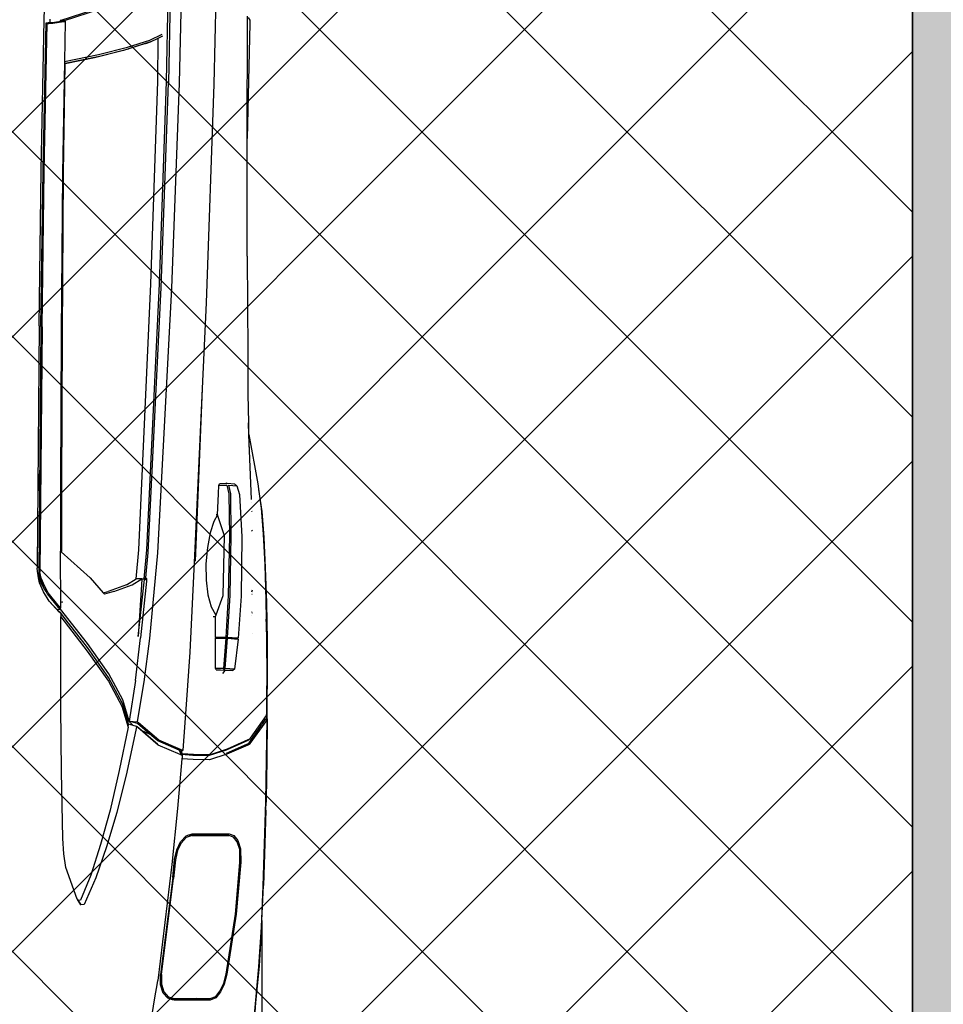
# Model space of a CAD drawing. Units: inches. Extents: x 2167 to 2589, y 1680 to 2489.
# Tile 18 of 38: x 2387 to 2419, y 1727 to 1761. Entities that reach past the tile are written whole.
import ezdxf

# ---------------------------------------------------------------- set-up
doc = ezdxf.new("R2010")
doc.units = ezdxf.units.IN
doc.header["$MEASUREMENT"] = 0
doc.layers.get('0').update_dxf_attribs({"color": 250})
doc.layers.add('A-FLOR-PATT', color=254, linetype='Continuous', lineweight=13, true_color=0xfeeab9)
for name, color, linetype, lineweight in [('C-PRKG-VEHS', 8, 'Continuous', 13), ('L-PVMT-PATT', 252, 'Continuous', 13), ('walls', 7, 'Continuous', 35)]:
    doc.layers.add(name, color=color, linetype=linetype, lineweight=lineweight)
doc.layers.add('Edges', color=250, linetype='Continuous')

# ---------------------------------------------------------------- blocks, each defined once
blk = doc.blocks.new('Nissan Qashqai pl')
at = {"layer": 'Edges'}
for p, q in [((10.4573, 12.8093), (10.4889, 12.8119)), ((10.4613, 12.8099), (10.4926, 12.8125)), ((10.4889, 12.8119), (10.526, 12.8138)), ((10.4926, 12.8125), (10.5294, 12.8143)), ((10.526, 12.8138), (10.569, 12.8151)), ((10.5294, 12.8143), (10.5719, 12.8156)), ((10.569, 12.8151), (10.5919, 12.8155)), ((10.5719, 12.8156), (10.6176, 12.8164)), ((10.5919, 12.8155), (10.6151, 12.8159)), ((10.5981, 12.8157), (10.5919, 12.8155)), ((10.6174, 12.816), (10.5981, 12.8157)), ((10.6151, 12.8159), (10.6644, 12.8162)), ((10.6176, 12.8164), (10.6651, 12.8167)), ((10.6644, 12.8162), (10.7078, 12.8159)), ((10.6651, 12.8167), (10.666, 12.8167)), ((10.666, 12.8167), (10.677, 12.8167)), ((10.6729, 12.8157), (10.7082, 12.8156)), ((10.6809, 12.8167), (10.677, 12.8167)), ((10.7128, 12.8166), (10.6809, 12.8167)), ((10.7078, 12.8159), (10.7083, 12.8156)), ((10.7082, 12.8156), (10.7078, 12.8159)), ((10.7085, 12.8153), (10.7082, 12.8156)), ((10.7082, 12.8156), (10.7083, 12.8156)), ((10.7083, 12.8156), (10.7087, 12.8153)), ((10.7083, 12.8156), (10.7125, 12.8156)), ((10.7087, 12.8153), (10.7363, 12.7959)), ((10.7139, 12.8164), (10.7125, 12.8156)), ((10.7137, 12.8148), (10.7125, 12.8156)), ((10.7128, 12.8166), (10.7625, 12.8161)), ((10.7128, 12.8166), (10.724, 12.8166)), ((10.7137, 12.8148), (10.7138, 12.8147)), ((10.7418, 12.7947), (10.7138, 12.8147)), ((10.7139, 12.8164), (10.7148, 12.8157)), ((10.7628, 12.8158), (10.7139, 12.8164)), ((10.7148, 12.8157), (10.7429, 12.7956)), ((10.7685, 12.8161), (10.724, 12.8166)), ((10.7625, 12.8161), (10.7628, 12.8161)), ((10.7628, 12.8161), (10.8099, 12.8152)), ((10.8131, 12.8149), (10.7628, 12.8158)), ((10.7688, 12.8161), (10.7685, 12.8161)), ((10.8099, 12.8152), (10.7688, 12.8161)), ((10.8099, 12.8152), (10.8131, 12.8152)), ((10.8134, 12.8152), (10.8131, 12.8152)), ((10.8644, 12.8135), (10.8131, 12.8149)), ((10.8134, 12.8152), (10.8142, 12.8152)), ((10.8142, 12.8152), (10.8142, 12.8152)), ((10.8237, 12.8149), (10.8142, 12.8152)), ((10.8237, 12.8149), (10.864, 12.8138)), ((10.8596, 12.8138), (10.8589, 12.8138)), ((10.8642, 12.8136), (10.8596, 12.8138)), ((10.864, 12.8138), (10.8642, 12.8138)), ((10.8642, 12.8138), (10.9152, 12.812)), ((10.9158, 12.8118), (10.8644, 12.8135)), ((10.9577, 12.8101), (10.9152, 12.812)), ((10.9657, 12.8095), (10.9158, 12.8118)), ((10.3679, 12.7944), (10.4275, 12.8051)), ((10.4275, 12.8051), (10.4304, 12.8056)), ((10.4304, 12.8056), (10.4339, 12.8061)), ((10.4339, 12.8061), (10.4573, 12.8093)), ((10.4339, 12.8061), (10.4345, 12.8062)), ((10.4345, 12.8062), (10.4613, 12.8099)), ((10.9577, 12.8101), (10.9649, 12.8097)), ((10.9577, 12.8101), (11.1283, 12.8101)), ((10.9649, 12.8097), (11.0127, 12.8067)), ((11.0138, 12.8064), (10.9657, 12.8095)), ((11.0127, 12.8067), (11.0576, 12.8026)), ((11.059, 12.8023), (11.0138, 12.8064)), ((11.0576, 12.8026), (11.0798, 12.8008)), ((11.0768, 12.8008), (11.059, 12.8023)), ((9.8643, 12.7927), (9.8598, 12.7928)), ((9.8614, 12.7937), (9.8647, 12.7956)), ((10.0085, 12.7922), (9.8643, 12.7927)), ((9.8647, 12.7956), (9.869, 12.7954)), ((9.869, 12.7954), (10.0085, 12.7922)), ((10.0124, 12.7922), (10.0085, 12.7922)), ((10.1513, 12.7924), (10.0124, 12.7922)), ((10.1513, 12.7924), (10.2677, 12.793)), ((10.2677, 12.793), (10.3189, 12.7931)), ((10.3189, 12.7931), (10.3537, 12.7939)), ((10.3537, 12.7939), (10.3832, 12.7945)), ((10.3679, 12.7944), (10.3537, 12.7939)), ((10.4468, 12.7976), (10.3679, 12.7944)), ((10.4503, 12.7976), (10.4502, 12.7976)), ((10.4603, 12.7976), (10.4613, 12.7978)), ((10.4838, 12.7977), (10.4852, 12.7982)), ((10.5565, 12.7985), (10.5591, 12.7977)), ((10.5615, 12.7978), (10.5617, 12.7985)), ((10.583, 12.7984), (10.5834, 12.798)), ((10.5836, 12.798), (10.5831, 12.7984)), ((10.5847, 12.798), (10.5841, 12.7984)), ((10.5873, 12.7981), (10.5873, 12.7981)), ((10.6087, 12.7983), (10.6087, 12.7984)), ((10.7363, 12.7959), (10.7376, 12.795)), ((10.7387, 12.794), (10.7376, 12.795)), ((10.7376, 12.795), (10.7378, 12.7946)), ((10.7378, 12.7946), (10.7379, 12.7945)), ((10.7378, 12.7946), (10.7385, 12.7932)), ((10.7385, 12.7932), (10.7497, 12.7679)), ((10.7387, 12.794), (10.7396, 12.7922)), ((10.7396, 12.7922), (10.7507, 12.7669)), ((10.743, 12.7939), (10.7418, 12.7947)), ((10.7432, 12.7954), (10.7426, 12.7954)), ((10.7429, 12.7956), (10.7432, 12.7954)), ((10.7434, 12.793), (10.743, 12.7939)), ((10.7441, 12.7954), (10.7432, 12.7954)), ((10.7432, 12.7954), (10.744, 12.7948)), ((10.7437, 12.7921), (10.7434, 12.793)), ((10.7438, 12.7921), (10.7437, 12.7921)), ((10.7438, 12.7921), (10.7549, 12.7666)), ((10.744, 12.7948), (10.7448, 12.793)), ((10.7448, 12.793), (10.7559, 12.7674)), ((10.4282, 12.7775), (10.4274, 12.7679)), ((10.4282, 12.7775), (10.4299, 12.7798)), ((10.4291, 12.77), (10.4299, 12.7798)), ((10.4299, 12.7798), (10.4406, 12.7829)), ((10.4406, 12.7829), (10.4919, 12.7858)), ((10.4919, 12.7858), (10.564, 12.7851)), ((10.564, 12.7851), (10.6151, 12.7813)), ((10.615, 12.7803), (10.6142, 12.7686)), ((10.6151, 12.7813), (10.615, 12.7803)), ((10.615, 12.7676), (10.6151, 12.7803)), ((10.6151, 12.7803), (10.615, 12.7803)), ((10.6151, 12.7803), (10.6151, 12.7813)), ((10.6151, 12.7685), (10.616, 12.7812)), ((10.616, 12.7812), (10.6526, 12.7768)), ((10.6526, 12.7768), (10.6518, 12.7657)), ((10.6526, 12.7768), (10.6543, 12.7749)), ((10.8523, 12.7704), (10.8546, 12.7762)), ((10.8546, 12.7762), (10.8607, 12.7808)), ((10.8622, 12.7801), (10.8565, 12.7757)), ((10.8607, 12.7808), (10.8708, 12.7841)), ((10.8716, 12.7832), (10.8622, 12.7801)), ((10.8708, 12.7841), (10.8869, 12.7844)), ((10.887, 12.7835), (10.8716, 12.7832)), ((10.8869, 12.7844), (10.9499, 12.7789)), ((10.9498, 12.7781), (10.887, 12.7835)), ((11.0226, 12.7668), (10.9498, 12.7781)), ((10.9499, 12.7789), (11.0229, 12.7676)), ((10.4263, 12.7665), (10.4274, 12.7674)), ((10.4274, 12.7679), (10.4274, 12.7674)), ((10.4274, 12.7674), (10.4275, 12.7586)), ((10.4398, 12.7724), (10.4291, 12.77)), ((10.4291, 12.7677), (10.4398, 12.7701)), ((10.4293, 12.7579), (10.4291, 12.7677)), ((10.4909, 12.773), (10.4398, 12.7724)), ((10.4398, 12.7701), (10.4909, 12.7708)), ((10.4908, 12.7648), (10.4653, 12.7564)), ((10.563, 12.7633), (10.4908, 12.7648)), ((10.5631, 12.7715), (10.4909, 12.773)), ((10.4909, 12.7708), (10.563, 12.7692)), ((10.563, 12.7692), (10.6142, 12.7663)), ((10.6142, 12.7686), (10.5631, 12.7715)), ((10.6142, 12.766), (10.6141, 12.7537)), ((10.6142, 12.7686), (10.6142, 12.7677)), ((10.6142, 12.7677), (10.615, 12.7676)), ((10.6142, 12.7677), (10.6142, 12.7663)), ((10.6142, 12.7663), (10.6142, 12.766)), ((10.6151, 12.7676), (10.615, 12.7676)), ((10.615, 12.7537), (10.6151, 12.7659)), ((10.6518, 12.7657), (10.6151, 12.7685)), ((10.6151, 12.7676), (10.6151, 12.7685)), ((10.6151, 12.7662), (10.6151, 12.7676)), ((10.6151, 12.7662), (10.6518, 12.7634)), ((10.6151, 12.7659), (10.6151, 12.7662)), ((10.6536, 12.7639), (10.6518, 12.7657)), ((10.6518, 12.7657), (10.6518, 12.7634)), ((10.6518, 12.7634), (10.6536, 12.7639)), ((10.6543, 12.7656), (10.6535, 12.7546)), ((10.6535, 12.7546), (10.6536, 12.7639)), ((10.6536, 12.7639), (10.6537, 12.7658)), ((10.6537, 12.7658), (10.6543, 12.7749)), ((10.6537, 12.7658), (10.6543, 12.7656)), ((10.6543, 12.7749), (10.6543, 12.7656)), ((10.6578, 12.7628), (10.6543, 12.7656)), ((10.7497, 12.7679), (10.7565, 12.7473)), ((10.7507, 12.7669), (10.7575, 12.7462)), ((10.7559, 12.7674), (10.7626, 12.7467)), ((10.8523, 12.7255), (10.8523, 12.7704)), ((10.8543, 12.7702), (10.8538, 12.753)), ((10.8565, 12.7757), (10.8543, 12.7702)), ((10.8543, 12.7255), (10.8543, 12.7702)), ((11.0339, 12.7639), (11.0226, 12.7668)), ((11.0229, 12.7676), (11.0348, 12.7645)), ((11.0429, 12.7597), (11.0339, 12.7639)), ((11.0348, 12.7645), (11.0444, 12.7601)), ((9.8024, 12.7549), (9.9426, 12.7518)), ((10.4293, 12.7579), (10.4275, 12.7586)), ((10.4398, 12.7573), (10.4293, 12.7579)), ((10.4653, 12.7564), (10.4398, 12.7573)), ((10.4653, 12.7561), (10.4652, 12.7545)), ((10.4653, 12.7564), (10.4653, 12.7561)), ((10.4653, 12.7564), (10.4653, 12.7564)), ((10.4653, 12.7564), (10.4653, 12.7561)), ((10.4653, 12.7561), (10.4653, 12.7561)), ((10.4653, 12.7561), (10.4732, 12.7517)), ((10.5867, 12.7545), (10.563, 12.7633)), ((10.5769, 12.7484), (10.5863, 12.7537)), ((10.5863, 12.7537), (10.5867, 12.7545)), ((10.5885, 12.7538), (10.5867, 12.7545)), ((10.5885, 12.751), (10.5885, 12.7538)), ((10.6141, 12.7537), (10.5885, 12.7538)), ((10.6141, 12.7537), (10.615, 12.7537)), ((10.6517, 12.754), (10.615, 12.7537)), ((10.6518, 12.7634), (10.6517, 12.754)), ((10.6535, 12.7546), (10.6517, 12.754)), ((10.8528, 12.7503), (10.8535, 12.7521)), ((10.8535, 12.7521), (10.8538, 12.753)), ((10.8538, 12.7521), (10.8535, 12.7521)), ((10.8538, 12.753), (10.8538, 12.7521)), ((10.8538, 12.7521), (10.8538, 12.7502)), ((11.0497, 12.7542), (11.0429, 12.7597)), ((11.0444, 12.7601), (11.0516, 12.7542)), ((11.0523, 12.7475), (11.0497, 12.7542)), ((11.0516, 12.7542), (11.0543, 12.7473)), ((9.9426, 12.7518), (10.2081, 12.7424)), ((10.2081, 12.7424), (10.312, 12.7377)), ((10.4732, 12.7517), (10.4871, 12.7474)), ((10.4871, 12.7474), (10.5048, 12.744)), ((10.5048, 12.744), (10.5246, 12.7423)), ((10.5246, 12.7423), (10.5445, 12.7425)), ((10.5445, 12.7425), (10.5625, 12.7446)), ((10.5625, 12.7446), (10.5769, 12.7484)), ((10.7565, 12.7473), (10.7563, 12.7273)), ((10.7575, 12.7462), (10.7572, 12.7263)), ((10.7626, 12.7467), (10.7623, 12.7269)), ((10.8528, 12.742), (10.8528, 12.7503)), ((10.8528, 12.742), (10.8538, 12.742)), ((10.8528, 12.7419), (10.8528, 12.742)), ((10.8538, 12.7419), (10.8528, 12.7419)), ((10.8528, 12.7242), (10.8528, 12.7419)), ((10.8538, 12.7502), (10.8538, 12.742)), ((10.8538, 12.742), (10.8538, 12.7419)), ((10.8538, 12.7214), (10.8538, 12.7419)), ((11.0528, 12.73), (11.0523, 12.7475)), ((11.0523, 12.7312), (11.0523, 12.7475)), ((11.0543, 12.7473), (11.0543, 12.7035)), ((10.312, 12.7377), (10.5214, 12.7293)), ((10.312, 12.7377), (10.5147, 12.7285)), ((10.5147, 12.7285), (10.6318, 12.7228)), ((11.0523, 12.7312), (11.0528, 12.73)), ((11.0523, 12.7287), (11.0523, 12.7312)), ((11.0528, 12.7274), (11.0523, 12.7287)), ((11.0523, 12.7037), (11.0523, 12.7287)), ((11.0528, 12.7274), (11.0528, 12.73)), ((11.0528, 12.73), (11.0538, 12.7273)), ((10.6318, 12.7228), (10.6955, 12.7184)), ((10.6955, 12.7184), (10.7509, 12.714)), ((10.7563, 12.7273), (10.7553, 12.7134)), ((10.7572, 12.7263), (10.7563, 12.7126)), ((10.7623, 12.7269), (10.7615, 12.7131)), ((10.8528, 12.7242), (10.8523, 12.7255)), ((10.8538, 12.7214), (10.8528, 12.7242)), ((10.855, 12.7181), (10.8538, 12.7214)), ((10.8543, 12.7255), (10.8569, 12.7184)), ((10.8622, 12.7114), (10.855, 12.7181)), ((10.8569, 12.7184), (10.8637, 12.712)), ((11.0528, 12.7274), (11.0528, 12.6985)), ((11.0538, 12.7273), (11.0538, 12.7018)), ((9.9414, 12.71), (9.8143, 12.713)), ((10.19, 12.7008), (9.9414, 12.71)), ((10.7501, 12.7114), (10.7387, 12.6849)), ((10.7507, 12.7098), (10.7397, 12.684)), ((10.7563, 12.7109), (10.7449, 12.6843)), ((10.7507, 12.7132), (10.7501, 12.7114)), ((10.7506, 12.7111), (10.7507, 12.7132)), ((10.7507, 12.7132), (10.7509, 12.714)), ((10.751, 12.7132), (10.7507, 12.7132)), ((10.7511, 12.7107), (10.7507, 12.7098)), ((10.7524, 12.7106), (10.7507, 12.7098)), ((10.7522, 12.7131), (10.7509, 12.714)), ((10.7516, 12.7131), (10.7509, 12.714)), ((10.7519, 12.7128), (10.7511, 12.7107)), ((10.7522, 12.7131), (10.7516, 12.7131)), ((10.7519, 12.7128), (10.7516, 12.7131)), ((10.7526, 12.7124), (10.7519, 12.7128)), ((10.7553, 12.7134), (10.7522, 12.7131)), ((10.7524, 12.7106), (10.7526, 12.7124)), ((10.7556, 12.7122), (10.7524, 12.7106)), ((10.7526, 12.7124), (10.7526, 12.7127)), ((10.7532, 12.712), (10.7526, 12.7124)), ((10.7556, 12.7122), (10.7532, 12.712)), ((10.7561, 12.7125), (10.7556, 12.7122)), ((10.7561, 12.7125), (10.7563, 12.7126)), ((10.7563, 12.7125), (10.7561, 12.7125)), ((10.7563, 12.7123), (10.7561, 12.7123)), ((10.7563, 12.7126), (10.7573, 12.7135)), ((10.7563, 12.7126), (10.7563, 12.7125)), ((10.7569, 12.7125), (10.7563, 12.7109)), ((10.7569, 12.7125), (10.7563, 12.7125)), ((10.7563, 12.7125), (10.7563, 12.7123)), ((10.7573, 12.7135), (10.7569, 12.7125)), ((10.7573, 12.7135), (10.7604, 12.7132)), ((10.7604, 12.7132), (10.7615, 12.7131)), ((10.7615, 12.7131), (10.8218, 12.7077)), ((10.8218, 12.7077), (10.8896, 12.7008)), ((10.8718, 12.7068), (10.8622, 12.7114)), ((10.8637, 12.712), (10.8727, 12.7077)), ((10.8836, 12.7041), (10.8718, 12.7068)), ((10.8727, 12.7077), (10.8839, 12.7051)), ((10.9054, 12.702), (10.8836, 12.7041)), ((10.8839, 12.7051), (10.9067, 12.7029)), ((9.8101, 12.6993), (9.9411, 12.6966)), ((9.9393, 12.6944), (9.8119, 12.697)), ((10.1849, 12.6857), (9.9393, 12.6944)), ((10.1894, 12.6879), (9.9411, 12.6966)), ((10.5113, 12.6839), (10.19, 12.7008)), ((10.8896, 12.7008), (11.0304, 12.6838)), ((10.9054, 12.702), (11.0232, 12.6871)), ((11.0231, 12.6882), (10.9067, 12.7029)), ((11.0443, 12.6911), (11.0501, 12.6964)), ((11.052, 12.6958), (11.0458, 12.6903)), ((11.0501, 12.6964), (11.0523, 12.7037)), ((11.0528, 12.6985), (11.052, 12.6958)), ((11.0538, 12.7018), (11.0528, 12.6985)), ((11.0543, 12.7035), (11.0538, 12.7018)), ((9.8891, 12.6741), (9.8818, 12.6891)), ((9.8867, 12.6842), (9.8838, 12.6901)), ((9.9393, 12.684), (9.8867, 12.6842)), ((9.8911, 12.675), (9.8867, 12.6842)), ((10.1849, 12.6754), (9.9393, 12.684)), ((10.5079, 12.6703), (10.1849, 12.6857)), ((10.5109, 12.6721), (10.1894, 12.6879)), ((10.6152, 12.674), (10.5113, 12.6839)), ((10.7387, 12.6849), (10.7177, 12.6604)), ((10.7449, 12.6843), (10.7232, 12.6594)), ((10.7438, 12.6836), (10.7265, 12.6635)), ((10.7397, 12.684), (10.7334, 12.6766)), ((11.0231, 12.6882), (11.035, 12.6883)), ((11.0358, 12.6872), (11.0232, 12.6871)), ((11.0357, 12.6829), (11.0304, 12.6838)), ((11.035, 12.6883), (11.0443, 12.6911)), ((11.0491, 12.6807), (11.0357, 12.6829)), ((11.0458, 12.6903), (11.0358, 12.6872)), ((11.0449, 12.6812), (11.0448, 12.6812)), ((11.0492, 12.6807), (11.0491, 12.6807)), ((11.1336, 12.667), (11.0492, 12.6807)), ((9.8978, 12.6472), (9.8891, 12.6741)), ((9.8911, 12.6749), (9.8911, 12.675)), ((9.8931, 12.6691), (9.8911, 12.6749)), ((9.8911, 12.6749), (9.8998, 12.6481)), ((9.8931, 12.669), (9.8931, 12.6691)), ((9.8931, 12.669), (9.9018, 12.6421)), ((10.5079, 12.6607), (10.1849, 12.6754)), ((10.543, 12.6671), (10.5079, 12.6703)), ((10.5417, 12.6693), (10.5109, 12.6721)), ((10.5417, 12.6693), (10.5427, 12.6702)), ((10.5417, 12.6693), (10.543, 12.6671)), ((10.5436, 12.6687), (10.5427, 12.6702)), ((10.5427, 12.6702), (10.5458, 12.67)), ((10.544, 12.6678), (10.5436, 12.6687)), ((10.5458, 12.67), (10.6144, 12.6629)), ((10.6678, 12.6672), (10.6152, 12.674)), ((10.7334, 12.6766), (10.7186, 12.6593)), ((10.7265, 12.6635), (10.7316, 12.6741)), ((10.543, 12.6576), (10.5079, 12.6607)), ((10.544, 12.6678), (10.543, 12.6671)), ((10.543, 12.6646), (10.543, 12.6671)), ((10.543, 12.6646), (10.543, 12.6576)), ((10.5439, 12.6646), (10.543, 12.6646)), ((10.5502, 12.6526), (10.543, 12.6646)), ((10.5502, 12.6456), (10.543, 12.6576)), ((10.5439, 12.6646), (10.613, 12.6601)), ((10.547, 12.6674), (10.544, 12.6678)), ((10.613, 12.6601), (10.547, 12.6674)), ((10.6664, 12.6566), (10.6144, 12.6629)), ((10.6664, 12.6566), (10.7155, 12.649)), ((10.7137, 12.6595), (10.6678, 12.6672)), ((10.7165, 12.6591), (10.7137, 12.6595)), ((10.7186, 12.6593), (10.7155, 12.649)), ((10.7155, 12.649), (10.7165, 12.6591)), ((10.7177, 12.6604), (10.7165, 12.6591)), ((10.7221, 12.6581), (10.7209, 12.654)), ((10.7232, 12.6594), (10.7221, 12.6581)), ((10.7221, 12.6581), (10.7224, 12.6587)), ((10.7221, 12.6581), (10.7247, 12.6575)), ((10.7265, 12.6635), (10.7224, 12.6587)), ((10.7247, 12.6575), (10.7776, 12.646)), ((9.9066, 12.6119), (9.8978, 12.6472)), ((9.9086, 12.6129), (9.8998, 12.6481)), ((10.5584, 12.6306), (10.5502, 12.6526)), ((10.5502, 12.6456), (10.5584, 12.6236)), ((10.7155, 12.649), (10.69, 12.6414)), ((10.7155, 12.6473), (10.6943, 12.641)), ((10.6976, 12.6401), (10.7228, 12.6477)), ((10.7209, 12.654), (10.7155, 12.6485)), ((10.7155, 12.649), (10.7155, 12.6485)), ((10.7155, 12.6485), (10.7155, 12.6473)), ((10.7192, 12.6484), (10.7155, 12.6473)), ((10.7209, 12.654), (10.7192, 12.6484)), ((10.7228, 12.6477), (10.7192, 12.6484)), ((10.7228, 12.6477), (10.7754, 12.637)), ((10.7776, 12.646), (10.8264, 12.6341)), ((9.9018, 12.6421), (9.9106, 12.6068)), ((10.69, 12.6414), (10.6583, 12.6245)), ((10.6943, 12.641), (10.6627, 12.6241)), ((10.6671, 12.6238), (10.6976, 12.6401)), ((10.7754, 12.637), (10.8239, 12.6261)), ((10.8264, 12.6341), (10.8682, 12.6216)), ((10.5584, 12.6306), (10.5617, 12.619)), ((10.56, 12.6176), (10.5584, 12.6236)), ((10.6583, 12.6245), (10.6215, 12.5986)), ((10.6627, 12.6241), (10.6261, 12.5984)), ((10.6306, 12.5982), (10.6671, 12.6238)), ((10.8239, 12.6261), (10.8653, 12.6144)), ((10.8682, 12.6216), (10.9059, 12.6087)), ((9.8652, 12.5704), (9.8516, 12.6129)), ((9.9149, 12.5705), (9.9066, 12.6119)), ((9.9169, 12.5714), (9.9086, 12.6129)), ((10.5419, 12.6018), (10.56, 12.6176)), ((10.56, 12.6176), (10.5617, 12.619)), ((10.8653, 12.6144), (10.9026, 12.6025)), ((10.9059, 12.6087), (10.9384, 12.5945)), ((9.8652, 12.5654), (9.8516, 12.6079)), ((9.9106, 12.6068), (9.9177, 12.5714)), ((10.51, 12.5666), (10.5419, 12.6018)), ((10.6215, 12.5986), (10.5796, 12.5655)), ((10.5892, 12.5659), (10.6306, 12.5982)), ((10.6261, 12.5984), (10.593, 12.5726)), ((10.9026, 12.6025), (10.933, 12.5901)), ((10.9316, 12.586), (10.8932, 12.572)), ((10.9316, 12.586), (10.9334, 12.5872)), ((10.932, 12.5862), (10.9316, 12.586)), ((10.9335, 12.5871), (10.932, 12.5862)), ((10.933, 12.5901), (10.9334, 12.5872)), ((10.9334, 12.5872), (10.9386, 12.5905)), ((10.9334, 12.5872), (10.9335, 12.5871)), ((10.9386, 12.5905), (10.9335, 12.5871)), ((10.9384, 12.5945), (10.9386, 12.5905)), ((9.8652, 12.5706), (9.8664, 12.5714)), ((9.8652, 12.5706), (9.8665, 12.5695)), ((9.8652, 12.5704), (9.8652, 12.5706)), ((9.8652, 12.5704), (9.8652, 12.5704)), ((9.8652, 12.5704), (9.8652, 12.5654)), ((9.8655, 12.5687), (9.8652, 12.5704)), ((9.8675, 12.5555), (9.8655, 12.5687)), ((9.8665, 12.5695), (9.8664, 12.5714)), ((9.8664, 12.5714), (9.9149, 12.5705)), ((9.8686, 12.5562), (9.8665, 12.5695)), ((9.9149, 12.5705), (10.0505, 12.5681)), ((9.9177, 12.5714), (9.9169, 12.5714)), ((10.0501, 12.5695), (9.9177, 12.5714)), ((10.2453, 12.568), (10.0501, 12.5695)), ((10.0505, 12.5681), (10.2453, 12.5664)), ((10.4292, 12.5674), (10.2453, 12.568)), ((10.2453, 12.5664), (10.4289, 12.5658)), ((10.4289, 12.5658), (10.5092, 12.5658)), ((10.5099, 12.5674), (10.4292, 12.5674)), ((10.5099, 12.5674), (10.5092, 12.5658)), ((10.5092, 12.5658), (10.5094, 12.5658)), ((10.5094, 12.5658), (10.51, 12.5666)), ((10.5783, 12.5659), (10.5094, 12.5658)), ((10.51, 12.5666), (10.5099, 12.5674)), ((10.5764, 12.5642), (10.5598, 12.5507)), ((10.5776, 12.5633), (10.5612, 12.5498)), ((10.5834, 12.5641), (10.57, 12.5517)), ((10.57, 12.5517), (10.5821, 12.5633)), ((10.5709, 12.5675), (10.5705, 12.5671)), ((10.5719, 12.5682), (10.5709, 12.5675)), ((10.5783, 12.5659), (10.5764, 12.5642)), ((10.5776, 12.5633), (10.5783, 12.5659)), ((10.5796, 12.5655), (10.5776, 12.5633)), ((10.5796, 12.5655), (10.5783, 12.5659)), ((10.5796, 12.562), (10.5796, 12.5655)), ((10.5838, 12.5653), (10.5821, 12.5633)), ((10.584, 12.5647), (10.5834, 12.5641)), ((10.584, 12.5655), (10.5838, 12.5653)), ((10.593, 12.5726), (10.584, 12.5655)), ((10.584, 12.5655), (10.5841, 12.5655)), ((10.584, 12.5654), (10.584, 12.5655)), ((10.5847, 12.5655), (10.584, 12.5647)), ((10.584, 12.5647), (10.584, 12.5654)), ((10.5851, 12.5659), (10.5841, 12.5655)), ((10.5841, 12.5655), (10.5847, 12.5655)), ((10.5851, 12.5659), (10.5847, 12.5655)), ((10.5851, 12.5659), (10.5892, 12.5659)), ((10.6988, 12.5662), (10.5892, 12.5659)), ((10.7769, 12.5667), (10.6988, 12.5662)), ((10.858, 12.5683), (10.7769, 12.5667)), ((10.8766, 12.5697), (10.858, 12.5683)), ((10.8932, 12.572), (10.8766, 12.5697)), ((9.8644, 12.5459), (9.696, 12.551)), ((9.8643, 12.5532), (9.8637, 12.5532)), ((9.8677, 12.5531), (9.8643, 12.5532)), ((9.8677, 12.5531), (9.8675, 12.5555)), ((9.8678, 12.5507), (9.8677, 12.5531)), ((9.8681, 12.5482), (9.8678, 12.5507)), ((9.8681, 12.5482), (9.869, 12.5496)), ((9.8689, 12.5515), (9.8686, 12.5562)), ((9.869, 12.5496), (9.8689, 12.5515)), ((10.0477, 12.5459), (9.869, 12.5496)), ((10.5598, 12.5507), (10.5522, 12.5465)), ((10.5612, 12.5498), (10.5583, 12.5481)), ((10.57, 12.5517), (10.5589, 12.5451)), ((10.0472, 12.5423), (9.8644, 12.5459)), ((10.0476, 12.5445), (9.8681, 12.5482)), ((10.2357, 12.5398), (10.0472, 12.5423)), ((10.2367, 12.5419), (10.0476, 12.5445)), ((10.2369, 12.5433), (10.0477, 12.5459)), ((10.2357, 12.5398), (10.53, 12.5373)), ((10.2367, 12.5419), (10.5351, 12.5392)), ((10.2369, 12.5433), (10.5348, 12.5406)), ((10.4153, 12.5384), (10.4176, 12.5384)), ((10.4176, 12.5384), (10.4181, 12.5384)), ((10.4181, 12.5384), (10.4552, 12.538)), ((10.4181, 12.5384), (10.4181, 12.5384)), ((10.4778, 12.5378), (10.53, 12.5373)), ((10.5301, 12.5373), (10.53, 12.5373)), ((10.5335, 12.5378), (10.5301, 12.5373)), ((10.5419, 12.5391), (10.5335, 12.5378)), ((10.5422, 12.542), (10.5348, 12.5406)), ((10.5418, 12.5405), (10.5351, 12.5392)), ((10.5424, 12.5406), (10.5418, 12.5405)), ((10.5419, 12.5391), (10.5463, 12.541)), ((10.5479, 12.54), (10.5419, 12.5391)), ((10.5522, 12.5465), (10.5422, 12.542)), ((10.5495, 12.5438), (10.5424, 12.5406)), ((10.5463, 12.541), (10.5551, 12.5457)), ((10.5589, 12.5451), (10.5479, 12.54)), ((10.5546, 12.546), (10.5495, 12.5438)), ((10.5583, 12.5481), (10.5546, 12.546)), ((10.5551, 12.5457), (10.5583, 12.5481))]:
    blk.add_line(p, q, dxfattribs=at)
blk = doc.blocks.new('car')
blk.add_blockref('Nissan Qashqai pl', (-9.7433, -11.9151))
blk = doc.blocks.new('carr')
blk.add_blockref('car', (0.5124, -0.007))

msp = doc.modelspace()

# ---------------------------------------------------------------- hatches: boundary and pattern name
at = {"layer": 'A-FLOR-PATT'}
h = msp.add_hatch(color=256, dxfattribs=at)
h.dxf.hatch_style = 1
h.paths.add_polyline_path([(2525.548, 1864.695), (2455.041, 1864.695), (2455.041, 1855.153), (2455.041, 1830.653), (2525.548, 1830.653)])
h.paths.add_polyline_path([(2455.041, 1855.153), (2452.048, 1855.153), (2452.048, 1864.695), (2426.208, 1864.695), (2422.048, 1864.695), (2422.048, 1788.195), (2467.347, 1788.195), (2467.347, 1812.195), (2452.048, 1812.195), (2452.048, 1830.653), (2455.041, 1830.653)])
h.paths.add_polyline_path([(2419.685, 1779.195), (2417.548, 1779.195), (2417.548, 1696.695), (2419.685, 1696.695)])
at = {"layer": 'L-PVMT-PATT'}
h = msp.add_hatch(dxfattribs=at)
h.set_pattern_fill('ANSI37', color=256, scale=40)
h.paths.add_polyline_path([(2417.548, 1783.695), (2417.548, 1846.042), (2239.361, 1846.042), (2239.361, 1687.695), (2369.843, 1687.695), (2369.843, 1696.695), (2375.607, 1696.695), (2416.107, 1696.695), (2417.548, 1696.695)])

# ---------------------------------------------------------------- linework, layer by layer
at = {"layer": 'walls'}
msp.add_line((2417.548, 1783.695), (2417.548, 1696.695), dxfattribs=at)

# ---------------------------------------------------------------- block references
at = {"layer": 'C-PRKG-VEHS', "xscale": 28.42784210623918, "yscale": 28.42784210623918, "zscale": 28.42784210623918, "rotation": 270}
msp.add_blockref('carr', (2369.852, 1779.037), dxfattribs=at)

doc.saveas('drawing.dxf')
